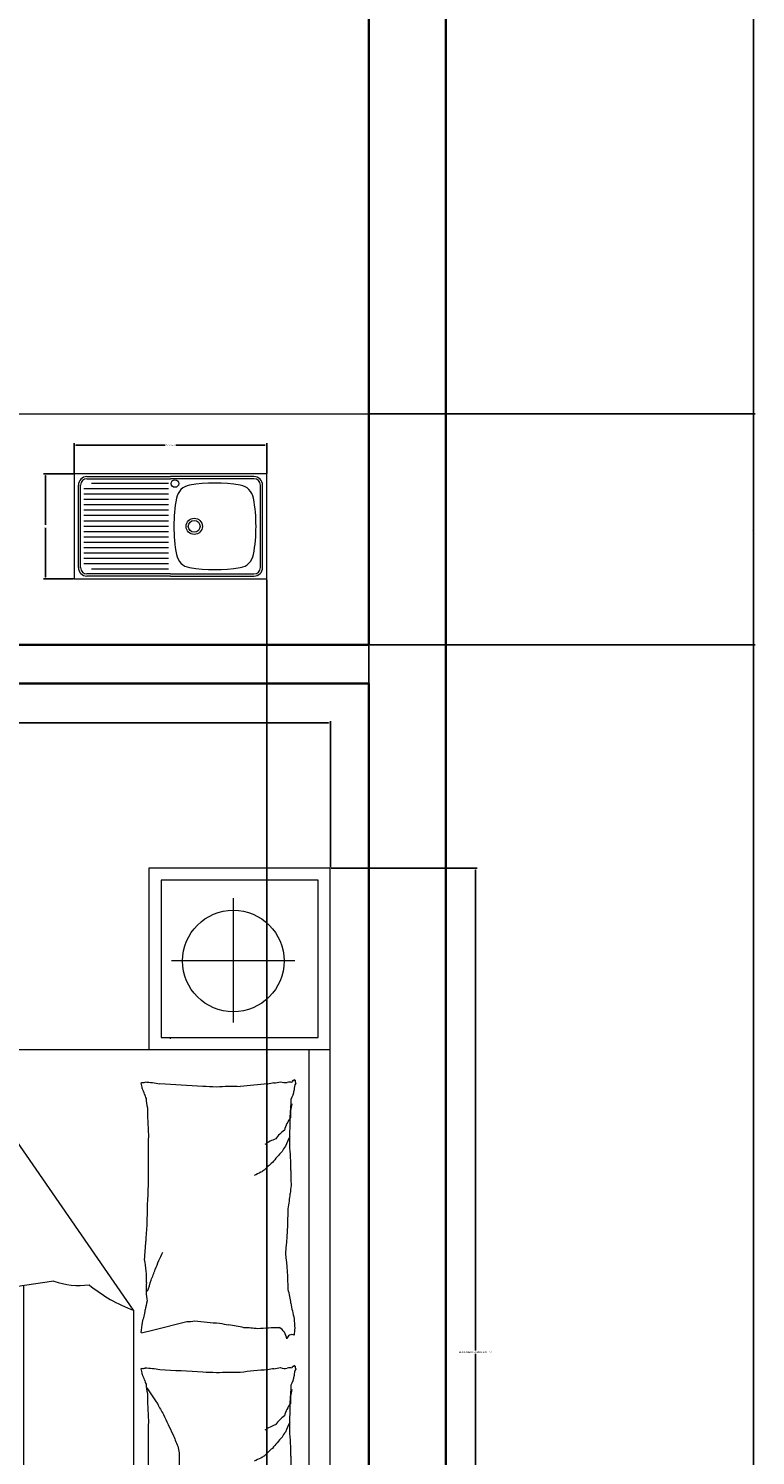
# Model space of a CAD drawing. Units: feet. Extents: x 1993 to 2298, y 2938 to 3641.
# Tile 7 of 11: x 2222 to 2298, y 3144 to 3293. Entities that reach past the tile are written whole.
import ezdxf

# ---------------------------------------------------------------- set-up
doc = ezdxf.new("R2010")
doc.units = ezdxf.units.FT
for name, color, linetype, lineweight in [('A-ANNO-DIMS', 2, 'Continuous', 18), ('A-FLOR-CASE', 8, 'Continuous', 18), ('A-FLOR-FIXT', 9, 'Continuous', 18), ('furniture', 8, 'Continuous', 18), ('WAL', 7, 'Continuous', 35)]:
    doc.layers.add(name, color=color, linetype=linetype, lineweight=lineweight)
doc.styles.add('DIM_FONT', font='SIMPLEX.shx', dxfattribs={"width": 0.8})
doc.styles.get("Standard").update_dxf_attribs({"font": 'arial.ttf'})
doc.dimstyles.get("Standard").update_dxf_attribs({"dimtxt": 0.18, "dimasz": 0.18, "dimexe": 0.18, "dimexo": 0.0625, "dimgap": 0.09, "dimtad": 0, "dimtih": 1, "dimtoh": 1, "dimdec": 4, "dimzin": 0, "dimdsep": 46, "dimtxsty": 'Standard', "dimcen": 0.09, "dimadec": 0, "dimazin": 0, "dimtfac": 1, "dimtdec": 4, "dimtofl": 0, "dimtmove": 0, "dimatfit": 3, "dimfxl": 1, "dimtolj": 1, "dimtzin": 0, "dimarcsym": 0})

# ---------------------------------------------------------------- blocks, each defined once
blk = doc.blocks.new('A$C79766A75')
for p, q in [((0.45, 1.9999), (0, 1.9999)), ((0, 1.9999), (0, 1.5499)), ((0.45, 1.5499), (0.45, 1.9999)), ((1.9506, 2), (0.4506, 2)), ((0.4506, 2), (0.4506, 0)), ((1.9506, 0), (1.9506, 2)), ((2.402, 1.9999), (1.952, 1.9999)), ((1.952, 1.9999), (1.952, 1.5499)), ((2.402, 1.5499), (2.402, 1.9999)), ((0.42, 1.9699), (0.03, 1.9699)), ((0.03, 1.9699), (0.03, 1.5799)), ((0.42, 1.5799), (0.42, 1.9699)), ((2.372, 1.9699), (1.982, 1.9699)), ((1.982, 1.9699), (1.982, 1.5799)), ((2.372, 1.5799), (2.372, 1.9699)), ((0.2304, 1.9125), (0.2304, 1.6061)), ((1.9506, 1.9476), (0.4506, 1.9476)), ((2.1824, 1.9125), (2.1824, 1.6061)), ((0.0743, 1.7595), (0.3834, 1.7595)), ((2.0263, 1.7595), (2.3354, 1.7595)), ((1.1461, 1.5617), (1.1254, 1.6443)), ((1.8553, 1.5617), (1.8346, 1.6443)), ((0.4234, 1.6034), (0.4228, 1.6034)), ((0.03, 1.5799), (0.42, 1.5799)), ((1.1536, 1.5317), (1.1461, 1.5617)), ((1.8628, 1.5317), (1.8553, 1.5617)), ((1.982, 1.5799), (2.372, 1.5799)), ((0, 1.5499), (0.45, 1.5499)), ((1.952, 1.5499), (2.402, 1.5499)), ((1.0972, 1.5115), (0.4791, 1.0841)), ((1.0972, 1.5115), (1.9048, 1.5115)), ((1.9248, 1.4915), (1.9248, 0.0322)), ((1.0383, 1.2184), (1.0246, 1.3138)), ((1.9048, 1.2389), (1.0354, 1.2389)), ((1.0365, 1.0883), (1.0383, 1.2184)), ((0.4791, 0.0622), (0.4791, 1.0841)), ((1.1731, 0.6316), (1.2523, 0.5276)), ((1.5696, 0.6317), (1.5559, 0.5286)), ((1.2523, 0.5276), (1.3274, 0.3973)), ((1.4223, 0.4407), (1.442, 0.5296)), ((1.5559, 0.5286), (1.5817, 0.4065)), ((1.6952, 0.4478), (1.7898, 0.4856)), ((1.7898, 0.4856), (1.8139, 0.4822)), ((1.4025, 0.3834), (1.4223, 0.4407)), ((1.6264, 0.355), (1.6952, 0.4478)), ((1.3274, 0.3973), (1.3452, 0.342)), ((1.5817, 0.4065), (1.6264, 0.355)), ((1.1139, 0.3597), (1.0779, 0.3397)), ((1.2167, 0.3736), (1.1139, 0.3597)), ((1.3452, 0.342), (1.2167, 0.3736)), ((1.3452, 0.342), (1.4025, 0.3834)), ((1.4034, 0.3558), (1.3803, 0.2995)), ((1.6264, 0.355), (1.4406, 0.3361)), ((1.5954, 0.2725), (1.6264, 0.355)), ((1.6264, 0.355), (1.6935, 0.3825)), ((1.6935, 0.3825), (1.7623, 0.379)), ((1.7623, 0.379), (1.8603, 0.3619)), ((1.8603, 0.3619), (1.8636, 0.3554)), ((1.2957, 0.2787), (1.3452, 0.342)), ((1.3452, 0.342), (1.3569, 0.2478)), ((1.4406, 0.3361), (1.3907, 0.3)), ((1.3803, 0.2995), (1.3626, 0.256)), ((1.3907, 0.3), (1.3787, 0.2914)), ((1.2305, 0.2313), (1.2957, 0.2787)), ((1.6161, 0.19), (1.5954, 0.2725)), ((1.1376, 0.2313), (1.2305, 0.2313)), ((1.3588, 0.2331), (1.3706, 0.1385)), ((1.6697, 0.1274), (1.6161, 0.19)), ((1.9048, 0.0122), (0.5291, 0.0122)), ((0.4506, 0), (1.9506, 0))]:
    blk.add_line(p, q)
for centre in [(0.2304, 1.7595), (2.1824, 1.7595)]:
    blk.add_circle(centre, 0.126)
for centre, radius, start, end in [((0.5232, 1.9139), 0.00342, 291.7883, 340.436), ((0.5246, 1.9378), 0.0251, 274.3025, 291.7883), ((0.5486, 1.9393), 0.0289, 239.3487, 274.3025), ((1.1179, 2.0719), 0.1611, 270, 278.4372), ((1.1592, 2.0011), 0.0904, 258.7276, 270), ((1.2325, 1.9139), 0.00342, 291.7883, 340.436), ((1.2338, 1.9378), 0.0251, 274.3025, 291.7883), ((1.2578, 1.9393), 0.0289, 239.3487, 274.3025), ((1.8271, 2.0719), 0.1611, 270, 278.4372), ((1.8684, 2.0011), 0.0904, 258.7276, 270), ((0.525, 1.9085), 0.00232, 340.436, 101.8931), ((0.5311, 1.9093), 0.00428, 201.9904, 281.8931), ((0.4996, 1.8889), 0.0328, 338.579, 8.1335), ((0.2896, 1.8253), 0.246, 8.1335, 12.1095), ((0.5465, 1.8994), 0.0156, 158.579, 201.9904), ((0.5458, 1.8568), 0.0539, 59.3487, 84.7408), ((0.546, 1.0829), 0.8208, 84.7408, 88.0921), ((0.6118, 2.0005), 0.0992, 254.0648, 274.2159), ((0.6775, 1.9817), 0.0992, 233.9136, 254.0648), ((0.6362, 0.406), 1.4943, 88.0921, 90.5757), ((0.7304, 1.9449), 0.0992, 216.1766, 233.9136), ((0.7737, 2.1075), 0.234, 242.7604, 249.1397), ((0.7591, 1.0293), 0.8732, 90.5757, 94.8018), ((0.738, 1.949), 0.0768, 231.6114, 242.7604), ((0.974, 2.1633), 0.3916, 226.1885, 231.6114), ((0.7631, 2.1919), 0.2897, 267.4614, 274.8018), ((0.8143, 2.0532), 0.1524, 259.8101, 267.4614), ((0.7515, 1.3747), 0.5293, 79.8101, 83.9133), ((0.8451, 0.8466), 1.049, 83.9133, 90), ((1.046, 1.2129), 0.6827, 90, 97.5469), ((1.1117, 1.6625), 0.2422, 97.5469, 105.744), ((1.0352, 2.2041), 0.3048, 278.4372, 285.744), ((1.171, 1.8579), 0.0342, 94.4002, 153.4195), ((1.1709, 1.9049), 0.0131, 153.4195, 258.7276), ((1.2342, 1.9085), 0.00232, 340.436, 101.8931), ((1.2404, 1.9093), 0.00428, 201.9904, 281.8931), ((1.2088, 1.8889), 0.0328, 338.579, 8.1335), ((0.9988, 1.8253), 0.246, 8.1335, 12.1095), ((1.2558, 1.8994), 0.0156, 158.579, 201.9904), ((1.2551, 1.8568), 0.0539, 59.3487, 84.7408), ((1.2552, 1.0829), 0.8208, 84.7408, 88.0921), ((1.3211, 2.0005), 0.0992, 254.0648, 274.2159), ((1.3868, 1.9817), 0.0992, 233.9136, 254.0648), ((1.3455, 0.406), 1.4943, 88.0921, 90.5757), ((1.4396, 1.9449), 0.0992, 216.1766, 233.9136), ((1.4829, 2.1075), 0.234, 242.7604, 249.1397), ((1.4683, 1.0293), 0.8732, 90.5757, 94.8018), ((1.4473, 1.949), 0.0768, 231.6114, 242.7604), ((1.6833, 2.1633), 0.3916, 226.1885, 231.6114), ((1.4724, 2.1919), 0.2897, 267.4614, 274.8018), ((1.5236, 2.0532), 0.1524, 259.8101, 267.4614), ((1.4607, 1.3747), 0.5293, 79.8101, 83.9133), ((1.5543, 0.8466), 1.049, 83.9133, 90), ((1.7552, 1.2129), 0.6827, 90, 97.5469), ((1.821, 1.6625), 0.2422, 97.5469, 105.744), ((1.7444, 2.2041), 0.3048, 278.4372, 285.744), ((1.8802, 1.8579), 0.0342, 94.4002, 153.4195), ((1.8802, 1.9049), 0.0131, 153.4195, 258.7276), ((0.7297, 1.8867), 0.1983, 187.6809, 192.1095), ((1.4472, 1.8987), 0.9131, 183.3687, 187.6809), ((0.7661, 1.8961), 0.0992, 198.4397, 216.1766), ((0.9057, 1.9982), 0.2252, 219.0349, 226.1885), ((1.6324, 1.8735), 0.4918, 180, 186.2324), ((1.4389, 1.8867), 0.1983, 187.6809, 192.1095), ((2.1565, 1.8987), 0.9131, 183.3687, 187.6809), ((1.4753, 1.8961), 0.0992, 198.4397, 216.1766), ((1.615, 1.9982), 0.2252, 219.0349, 226.1885), ((1.6908, 1.9123), 0.1399, 314.9024, 332.6012), ((1.7511, 1.9723), 0.1399, 297.2036, 314.9024), ((1.7896, 1.8667), 0.0526, 318.5571, 334.6449), ((1.784, 1.9167), 0.0899, 306.2641, 318.5571), ((2.3416, 1.8735), 0.4918, 180, 186.2324), ((0.7932, 1.8591), 0.0493, 208.3168, 219.0349), ((0.9392, 1.9062), 0.2002, 203.0028, 208.3168), ((1.3446, 1.7858), 0.204, 170.3156, 180), ((1.5025, 1.8591), 0.0493, 208.3168, 219.0349), ((1.6484, 1.9062), 0.2002, 203.0028, 208.3168), ((1.6554, 1.8529), 0.1399, 332.6012, 343.485), ((1.7653, 1.8132), 0.0562, 341.2201, 0), ((1.6307, 1.8895), 0.2056, 338.1851, 341.2201), ((1.6887, 1.8881), 0.1511, 334.6449, 338.1851), ((2.0538, 1.7858), 0.204, 170.3156, 180), ((1.2208, 1.7573), 0.6787, 178.3669, 183.3687), ((2.0027, 1.5994), 0.882, 167.8016, 170.3156), ((1.9301, 1.7573), 0.6787, 178.3669, 183.3687), ((1.6404, 1.8023), 0.1399, 343.485, 354.3689), ((1.73, 1.7719), 0.0915, 0, 14.6851), ((2.7119, 1.5994), 0.882, 167.8016, 170.3156), ((0.8192, 1.792), 0.3171, 347.8016, 351.9949), ((1.5284, 1.792), 0.3171, 347.8016, 351.9949), ((1.9066, 1.6447), 1.3652, 176.945, 178.3669), ((0.4711, 1.7556), 0.6588, 351.9949, 357.3351), ((2.6158, 1.6447), 1.3652, 176.945, 178.3669), ((1.1803, 1.7556), 0.6588, 351.9949, 357.3351), ((14.1519, 0.85), 13.6356, 176.49514, 176.94504), ((14.8612, 0.85), 13.6356, 176.49514, 176.94504), ((1.0578, 1.6474), 0.0677, 357.3351, 14.0452), ((1.767, 1.6474), 0.0677, 357.3351, 14.0452), ((0.7658, 2.8912), 1.4323, 294.3265, 296.4985), ((1.226, 2.0834), 0.5066, 290.6743, 294.3265), ((1.4305, 1.6796), 0.058, 274.0828, 290.6743), ((1.4679, 1.8969), 0.2721, 266.4448, 274.0828), ((0.8521, 1.5209), 0.3212, 170.0016, 176.4951), ((0.6583, 0.9067), 0.7387, 64.6889, 66.5156), ((0.7015, 0.888), 0.7387, 66.5156, 68.3423), ((0.7501, 0.8688), 0.7387, 68.3423, 70.572), ((1.5613, 1.5209), 0.3212, 170.0016, 176.4951), ((0.9025, 2.1618), 0.7286, 302.135, 305.8263), ((1.1895, 1.8508), 0.3126, 296.4985, 302.135), ((1.3675, 0.9067), 0.7387, 64.6889, 66.5156), ((1.4107, 0.888), 0.7387, 66.5156, 68.3423), ((1.4594, 0.8688), 0.7387, 68.3423, 70.572), ((0.513, 1.535), 0.0193, 350.0016, 16.6978), ((0.5322, 1.5304), 0.00132, 16.6978, 97.1204), ((0.5579, 1.4467), 0.0875, 97.1204, 106.2212), ((0.5822, 1.4654), 0.0767, 106.2212, 117.2841), ((0.5507, 1.5832), 0.0453, 282.869, 297.2841), ((0.5623, 1.6885), 0.1459, 273.574, 282.869), ((0.589, 2.7103), 1.164, 270.2865, 273.574), ((0.7584, 7.2662), 5.7185, 269.0296, 270.2865), ((0.9401, 4.9065), 3.3622, 267.3904, 269.0296), ((0.9811, 2.7573), 1.2165, 265.3824, 267.3904), ((0.8583, 0.139), 1.4048, 85.3824, 87.2509), ((1.0175, 1.3138), 0.2301, 87.2509, 101.5586), ((0.8043, 0.8497), 0.7387, 70.572, 72.8018), ((1.0449, 1.6886), 0.1459, 263.5659, 281.5586), ((1.1099, 1.6599), 0.1197, 252.6136, 263.5659), ((1.0587, 1.3144), 0.2297, 72.6136, 80.5159), ((1.108, 1.2635), 0.2708, 80.5159, 85.9171), ((1.1535, 1.5308), 0.000917, 85.9171, 194.0449), ((1.2222, 1.535), 0.0193, 350.0016, 16.6978), ((1.2414, 1.5304), 0.00132, 16.6978, 97.1204), ((1.2671, 1.4467), 0.0875, 97.1204, 106.2212), ((1.2914, 1.4654), 0.0767, 106.2212, 117.2841), ((1.2599, 1.5832), 0.0453, 282.869, 297.2841), ((1.2716, 1.6885), 0.1459, 273.574, 282.869), ((1.2982, 2.7103), 1.164, 270.2865, 273.574), ((1.4677, 7.2662), 5.7185, 269.0296, 270.2865), ((1.6493, 4.9065), 3.3622, 267.3904, 269.0296), ((1.6903, 2.7573), 1.2165, 265.3824, 267.3904), ((1.5676, 0.139), 1.4048, 85.3824, 87.2509), ((1.7268, 1.3138), 0.2301, 87.2509, 101.5586), ((1.5136, 0.8497), 0.7387, 70.572, 72.8018), ((1.7541, 1.6886), 0.1459, 263.5659, 281.5586), ((1.8192, 1.6599), 0.1197, 252.6136, 263.5659), ((1.7679, 1.3144), 0.2297, 72.6136, 80.5159), ((1.8172, 1.2635), 0.2708, 80.5159, 85.9171), ((1.8627, 1.5308), 0.000917, 85.9171, 194.0449), ((0.745, 1.6407), 0.3751, 320.3555, 339.8512), ((1.9048, 1.4915), 0.02, 0, 90), ((0.8556, 1.3759), 0.1801, 339.8512, 8.1356), ((1.9048, 1.2589), 0.02, 270, 0), ((-0.1888, 5.1029), 4.0646, 280.7276, 282.9255), ((0.7282, 1.1989), 0.0581, 262.2696, 280.7276), ((0.7833, 1.3309), 0.1942, 256.8096, 262.2696), ((0.2481, -1.3253), 2.5158, 76.8096, 78.3259), ((-0.0248, 2.8487), 1.8351, 285.9352, 287.7364), ((0.3872, 1.7415), 0.6574, 282.9255, 285.9352), ((0.3953, -1.4284), 2.588, 78.3259, 80.505), ((0.413, -2.64), 3.7801, 80.505, 82.308), ((1.1752, 0.6267), 0.0063, 166.7192, 233.4208), ((1.1734, 0.6272), 0.00443, 93.9484, 166.7192), ((1.163, 0.6103), 0.0142, 10.4074, 53.4208), ((1.1755, 0.5964), 0.0352, 69.6548, 93.9484), ((1.1011, 0.5989), 0.0771, 2.7286, 10.4074), ((1.1628, 0.6019), 0.0153, 345.4291, 2.7286), ((1.1669, 0.5731), 0.0601, 51.4146, 69.6548), ((1.2538, 0.682), 0.0792, 231.4146, 247.2931), ((1.5463, 1.3811), 0.8371, 247.2931, 249.8713), ((1.383, 0.7705), 0.2176, 307.2151, 313.5224), ((1.1426, 1.1456), 0.6605, 306.2163, 307.2151), ((1.7751, 0.3162), 0.3825, 126.2163, 127.5287), ((1.5806, 0.5924), 0.0452, 127.5287, 134.1274), ((1.5093, 0.6825), 0.0697, 308.8136, 314.1274), ((1.5706, 0.6318), 0.0127, 176.7545, 308.8136), ((1.5621, 0.59), 0.0359, 356.7545, 62.7098), ((0.9961, 0.6678), 0.194, 320.2995, 329.0944), ((0.8605, 0.749), 0.352, 329.0944, 333.1821), ((1.1396, 0.6079), 0.0393, 333.1821, 345.4291), ((3.0113, 5.3783), 5.0942, 249.8713, 250.9164), ((1.5435, 0.5526), 0.0458, 157.5838, 188.0492), ((1.4828, 0.5833), 0.0226, 324.1064, 8.0492), ((1.4519, 0.6426), 0.0774, 313.5224, 324.1064), ((0.2201, -2.1858), 3.0972, 62.7098, 63.5853), ((2.5711, 2.3551), 2.0162, 242.5001, 243.5853), ((1.2077, 0.4922), 0.081, 140.2995, 153.9265), ((2.374, 3.5362), 3.145, 250.9164, 253.3915), ((2.4089, 0.1204), 1.0054, 154.9471, 157.5838), ((4.5245, 5.9445), 6.1019, 242.15178, 242.50014), ((-0.9881, -4.647), 5.8383, 62.15178, 62.50792), ((3.0311, -0.112), 2.003, 162.1604, 164.7375), ((1.3115, 0.4414), 0.1965, 153.9265, 162.1604), ((2.9813, -0.2643), 1.6868, 152.9116, 154.9471), ((1.5084, 0.6341), 0.1166, 253.3915, 259.2634), ((1.5182, -0.068), 0.6236, 62.5079, 69.2514), ((1.7121, 0.0657), 0.43, 69.2514, 77.3748), ((1.8682, 0.4049), 0.063, 77.3748, 93.3881), ((1.8955, 0.5247), 0.0599, 256.9598, 273.3881), ((1.9257, 0.5082), 0.0509, 238.3083, 256.9598), ((2.8096, -0.3311), 1.5652, 150.064, 152.9116), ((1.8435, 0.4743), 0.0755, 310.5086, 333.6668), ((1.9279, 0.441), 0.0168, 130.5086, 180.9614), ((1.9201, 0.4587), 0.0058, 180.9614, 238.3083), ((2.6887, -0.0186), 1.6481, 164.7375, 166.159), ((-0.5166, 1.5491), 2.6619, 333.6668, 334.8268), ((0.5589, 0.5062), 0.5454, 343.6878, 346.159), ((1.2176, 0.4627), 0.2143, 330.064, 337.7645), ((1.3456, 0.5261), 0.5454, 339.2919, 341.7631), ((1.701, 0.4319), 0.1798, 334.8268, 339.2919), ((-1.4109, 1.284), 2.6619, 338.0627, 339.2227), ((0.9098, 0.4035), 0.1798, 339.2227, 343.6878), ((3.4079, -0.2212), 1.6481, 160.3416, 161.7631), ((0.9882, 0.3177), 0.0755, 314.9045, 338.0627), ((3.6966, -0.4634), 2.003, 157.7645, 160.3416), ((1.0533, 0.2524), 0.0168, 134.9045, 185.3572), ((1.0424, 0.2513), 0.0058, 185.3572, 242.7041), ((1.3694, 0.234), 0.0231, 107.1867, 157.7645), ((1.0631, 0.2914), 0.0509, 242.7041, 261.3557), ((1.0645, 0.3003), 0.0599, 261.3557, 277.784), ((1.0811, 0.1786), 0.063, 81.7707, 97.784), ((1.0286, -0.1846), 0.43, 73.6473, 81.7707), ((0.974, -0.3705), 0.6236, 66.9038, 73.6473), ((1.3465, 0.2383), 0.00467, 287.1867, 70.6201), ((1.3486, 0.2247), 0.0092, 70.6201, 94.2593), ((1.3563, 0.267), 0.034, 262.0178, 274.2593), ((1.4091, 0.4221), 0.1955, 255.1193, 262.0178), ((1.358, 0.0507), 0.1794, 75.1193, 82.3216), ((1.4096, 0.153), 0.0712, 82.3216, 94.5118), ((1.4285, 0.2893), 0.0663, 261.8784, 274.5118), ((1.4755, 0.332), 0.1166, 248.9957, 261.8784), ((2.7121, 3.1012), 3.145, 246.5205, 248.9957), ((2.4175, -0.1202), 1.0054, 160.6552, 161.9797), ((-1.0716, -5.1672), 5.8383, 66.54766, 66.9038), ((3.6805, 5.7866), 6.1019, 246.54766, 246.89602), ((1.505, 0.1766), 0.0458, 161.9797, 192.4451), ((1.856, 0.1288), 0.081, 135.9036, 149.5306), ((1.9797, 0.1108), 0.1965, 149.5306, 157.7645), ((2.0773, 2.0287), 2.0162, 246.896, 247.9812), ((0.1602, -2.7118), 3.0972, 67.1056, 67.9812), ((1.3914, 0.1905), 0.0774, 317.9183, 328.5023), ((1.4382, 0.1619), 0.0226, 328.5023, 12.4451), ((3.6993, 4.7998), 5.0942, 245.4754, 246.5205), ((1.4661, 0.3294), 0.352, 324.6985, 328.7862), ((1.6279, 0.2819), 0.194, 315.9036, 324.6985), ((1.3512, 0.1084), 0.0359, 1.1504, 67.1056), ((1.3997, 0.1094), 0.0127, 181.1504, 313.2095), ((1.4468, 0.0748), 0.0452, 131.9246, 138.5233), ((1.6722, -0.1762), 0.3825, 130.6122, 131.9246), ((0.9933, 0.6156), 0.6605, 310.6122, 311.611), ((1.2874, 0.2845), 0.2176, 311.611, 317.9183), ((2.051, 0.8725), 0.8371, 242.8972, 245.4754), ((1.7576, 0.1689), 0.0792, 227.0187, 242.8972), ((1.7345, 0.1188), 0.0153, 341.0332, 358.3327), ((1.6723, 0.1058), 0.0771, 358.3327, 6.0115), ((1.7162, 0.1388), 0.0393, 328.7862, 341.0332), ((1.3607, 0.1509), 0.0697, 313.2095, 318.5233), ((1.6963, 0.0438), 0.0601, 47.0187, 65.2589), ((1.737, 0.0526), 0.0352, 65.2589, 89.5525), ((1.7401, 0.0928), 0.0142, 6.0115, 49.0249), ((1.756, 0.0832), 0.00443, 89.5525, 162.3233), ((1.7602, 0.0924), 0.0063, 162.3233, 229.0249), ((0.5291, 0.0622), 0.05, 180, 270), ((1.9048, 0.0322), 0.02, 270, 0)]:
    blk.add_arc(centre, radius, start, end)
at = {"style": 'DIM_FONT', "text_generation_flag": 4, "width": 0.8, "flags": 9}
for tag in ['XSIZE', 'YSIZE']:
    blk.add_attdef(tag, (1.9506, 2), '', height=0.0005, rotation=180, dxfattribs=at)
blk = doc.blocks.new('A$C0C3933DC')
for p, q in [((0, 490), (0, 0)), ((900, 490), (0, 490)), ((59.5, 477.5), (450, 477.5)), ((59.5, 467.5), (450, 467.5)), ((840.5, 477.5), (450, 477.5)), ((840.5, 467.5), (450, 467.5)), ((900, 0), (900, 490)), ((19.5, 52.5), (19.5, 437.5)), ((29.5, 52.5), (29.5, 437.5)), ((441, 420), (45, 420)), ((441, 445), (80.7, 445)), ((870.5, 52.5), (870.5, 437.5)), ((880.5, 52.5), (880.5, 437.5)), ((441, 395), (45, 395)), ((441, 370), (45, 370)), ((441, 345), (45, 345)), ((441, 320), (45, 320)), ((441, 295), (45, 295)), ((441, 270), (45, 270)), ((441, 245), (45, 245)), ((441, 220), (45, 220)), ((441, 195), (45, 195)), ((441, 170), (45, 170)), ((441, 145), (45, 145)), ((441, 120), (45, 120)), ((441, 95), (45, 95)), ((441, 70), (45, 70)), ((0, 0), (900, 0)), ((450, 22.5), (59.5, 22.5)), ((450, 12.5), (59.5, 12.5)), ((441, 45), (80.7, 45)), ((450, 22.5), (840.5, 22.5)), ((450, 12.5), (840.5, 12.5))]:
    blk.add_line(p, q)
for centre, radius in [((471, 445), 17.5), ((561, 245), 38), ((561, 245), 27.5)]:
    blk.add_circle(centre, radius)
for centre, radius, start, end in [((59.5, 437.5), 40, 90, 180), ((59.5, 437.5), 30, 90, 180), ((840.5, 437.5), 40, 0, 90), ((840.5, 437.5), 30, 0, 90), ((551.5, 363.5), 75, 99.07872, 169.88522), ((658, -303), 750, 80.92128, 99.07872), ((764.5, 363.5), 75, 10.11478, 80.92128), ((1216, 245), 750, 169.88522, 190.11478), ((100, 245), 750, 349.88522, 10.11478), ((551.5, 126.5), 75, 190.11478, 260.92128), ((764.5, 126.5), 75, 279.07872, 349.88522), ((59.5, 52.5), 40, 180, 270), ((59.5, 52.5), 30, 180, 270), ((658, 793), 750, 260.92128, 279.07872), ((840.5, 52.5), 30, 270, 0), ((840.5, 52.5), 40, 270, 0)]:
    blk.add_arc(centre, radius, start, end)
blk = doc.blocks.new('*D30')
at = {"layer": 'A-ANNO-DIMS', "color": 0, "lineweight": -2, "transparency": 16777216}
for p, q in [((2253.83, 3205.36), (2269.02, 3205.36)), ((2268.84, 3205.18), (2268.84, 3155.29)), ((2268.84, 3105.04), (2268.84, 3154.93)), ((2253.83, 3104.86), (2269.02, 3104.86))]:
    blk.add_line(p, q, dxfattribs=at)
at = {"layer": 'A-ANNO-DIMS', "color": 0, "transparency": 16777216}
for points in [[(2268.81, 3205.18), (2268.87, 3205.18), (2268.84, 3205.36)], [(2268.81, 3105.04), (2268.87, 3105.04), (2268.84, 3104.86)]]:
    blk.add_solid(points, dxfattribs=at)
at = {"layer": 'Defpoints', "color": 0, "transparency": 16777216}
for p in [(2253.76, 3205.36), (2253.76, 3104.86), (2268.84, 3104.86)]:
    blk.add_point(p, dxfattribs=at)
at = {"layer": 'A-ANNO-DIMS', "color": 0, "transparency": 16777216, "insert": (2268.84, 3155.11), "char_height": 0.18, "attachment_point": 5}
blk.add_mtext('\\A1;BED & NIGHTSTANDS 100 TYP.', dxfattribs=at)
blk = doc.blocks.new('*D31')
at = {"layer": 'A-ANNO-DIMS', "color": 0, "lineweight": -2, "transparency": 16777216}
for p, q in [((2170.07, 3205.42), (2170.07, 3220.61)), ((2170.25, 3220.43), (2211.39, 3220.43)), ((2253.58, 3220.43), (2212.44, 3220.43)), ((2253.76, 3205.42), (2253.76, 3220.61))]:
    blk.add_line(p, q, dxfattribs=at)
at = {"layer": 'A-ANNO-DIMS', "color": 0, "transparency": 16777216}
for points in [[(2170.25, 3220.46), (2170.25, 3220.4), (2170.07, 3220.43)], [(2253.58, 3220.46), (2253.58, 3220.4), (2253.76, 3220.43)]]:
    blk.add_solid(points, dxfattribs=at)
at = {"layer": 'Defpoints', "color": 0, "transparency": 16777216}
for p in [(2253.76, 3220.43), (2170.07, 3205.36), (2253.76, 3205.36)]:
    blk.add_point(p, dxfattribs=at)
at = {"layer": 'A-ANNO-DIMS', "color": 0, "transparency": 16777216, "insert": (2211.92, 3220.43), "char_height": 0.18, "attachment_point": 5}
blk.add_mtext('\\A1;84 TYP.', dxfattribs=at)
blk = doc.blocks.new('*D52')
at = {"layer": 'A-ANNO-DIMS', "color": 0, "lineweight": -2, "transparency": 16777216}
for p, q in [((2227.15, 3246.35), (2227.15, 3249.47)), ((2227.33, 3249.29), (2236.6, 3249.29)), ((2246.97, 3249.29), (2237.7, 3249.29)), ((2247.15, 3246.35), (2247.15, 3249.47))]:
    blk.add_line(p, q, dxfattribs=at)
at = {"layer": 'A-ANNO-DIMS', "color": 0, "transparency": 16777216}
for points in [[(2227.33, 3249.32), (2227.33, 3249.26), (2227.15, 3249.29)], [(2246.97, 3249.32), (2246.97, 3249.26), (2247.15, 3249.29)]]:
    blk.add_solid(points, dxfattribs=at)
at = {"layer": 'Defpoints', "color": 0, "transparency": 16777216}
for p in [(2247.15, 3249.29), (2227.15, 3246.29), (2247.15, 3246.29)]:
    blk.add_point(p, dxfattribs=at)
at = {"layer": 'A-ANNO-DIMS', "color": 0, "transparency": 16777216, "insert": (2237.15, 3249.29), "char_height": 0.18, "attachment_point": 5}
blk.add_mtext('\\A1;SINK 20', dxfattribs=at)
blk = doc.blocks.new('*D53')
at = {"layer": 'A-ANNO-DIMS', "color": 0, "lineweight": -2, "transparency": 16777216}
for p, q in [((2227.09, 3246.29), (2223.97, 3246.29)), ((2224.15, 3246.11), (2224.15, 3241.02)), ((2224.15, 3235.58), (2224.15, 3240.66)), ((2227.09, 3235.4), (2223.97, 3235.4))]:
    blk.add_line(p, q, dxfattribs=at)
at = {"layer": 'A-ANNO-DIMS', "color": 0, "transparency": 16777216}
for points in [[(2224.12, 3246.11), (2224.18, 3246.11), (2224.15, 3246.29)], [(2224.12, 3235.58), (2224.18, 3235.58), (2224.15, 3235.4)]]:
    blk.add_solid(points, dxfattribs=at)
at = {"layer": 'Defpoints', "color": 0, "transparency": 16777216}
for p in [(2224.15, 3246.29), (2227.15, 3246.29), (2227.15, 3235.4)]:
    blk.add_point(p, dxfattribs=at)
at = {"layer": 'A-ANNO-DIMS', "color": 0, "transparency": 16777216, "insert": (2224.15, 3240.84), "char_height": 0.18, "attachment_point": 5}
blk.add_mtext('\\A1;11', dxfattribs=at)
blk = doc.blocks.new('*D55')
at = {"layer": 'A-ANNO-DIMS', "color": 0, "lineweight": -2, "transparency": 16777216}
for p, q in [((2265.82, 3608.53), (2297.9, 3608.53)), ((2297.72, 3608.35), (2297.72, 3308.72)), ((2297.72, 3008.71), (2297.72, 3308.35)), ((2265.82, 3008.53), (2297.9, 3008.53))]:
    blk.add_line(p, q, dxfattribs=at)
at = {"layer": 'A-ANNO-DIMS', "color": 0, "transparency": 16777216}
for points in [[(2297.69, 3608.35), (2297.75, 3608.35), (2297.72, 3608.53)], [(2297.69, 3008.71), (2297.75, 3008.71), (2297.72, 3008.53)]]:
    blk.add_solid(points, dxfattribs=at)
at = {"layer": 'Defpoints', "color": 0, "transparency": 16777216}
for p in [(2265.76, 3608.53), (2297.72, 3608.53), (2265.76, 3008.53)]:
    blk.add_point(p, dxfattribs=at)
at = {"layer": 'A-ANNO-DIMS', "color": 0, "transparency": 16777216, "insert": (2297.72, 3308.53), "char_height": 0.18, "attachment_point": 5}
blk.add_mtext('\\A1;600', dxfattribs=at)
blk = doc.blocks.new('*D61')
at = {"layer": 'A-ANNO-DIMS', "color": 0, "lineweight": -2, "transparency": 16777216}
for p, q in [((2257.82, 3252.53), (2297.9, 3252.53)), ((2297.72, 3252.35), (2297.72, 3240.71)), ((2297.72, 3228.71), (2297.72, 3240.35)), ((2257.82, 3228.53), (2297.9, 3228.53))]:
    blk.add_line(p, q, dxfattribs=at)
at = {"layer": 'A-ANNO-DIMS', "color": 0, "transparency": 16777216}
for points in [[(2297.69, 3252.35), (2297.75, 3252.35), (2297.72, 3252.53)], [(2297.69, 3228.71), (2297.75, 3228.71), (2297.72, 3228.53)]]:
    blk.add_solid(points, dxfattribs=at)
at = {"layer": 'Defpoints', "color": 0, "transparency": 16777216}
for p in [(2257.76, 3252.53), (2297.72, 3252.53), (2257.76, 3228.53)]:
    blk.add_point(p, dxfattribs=at)
at = {"layer": 'A-ANNO-DIMS', "color": 0, "transparency": 16777216, "insert": (2297.72, 3240.53), "char_height": 0.18, "attachment_point": 5}
blk.add_mtext('\\A1;24', dxfattribs=at)
blk = doc.blocks.new('*D66')
at = {"layer": 'A-ANNO-DIMS', "color": 0, "lineweight": -2, "transparency": 16777216}
for p, q in [((2247.15, 3235.34), (2247.15, 2937.86)), ((2257.76, 3228.47), (2257.76, 2937.86)), ((2247.33, 2938.03), (2252, 2938.03)), ((2257.58, 2938.03), (2252.91, 2938.03))]:
    blk.add_line(p, q, dxfattribs=at)
at = {"layer": 'A-ANNO-DIMS', "color": 0, "transparency": 16777216}
for points in [[(2247.33, 2938.07), (2247.33, 2938.01), (2247.15, 2938.03)], [(2257.58, 2938.07), (2257.58, 2938.01), (2257.76, 2938.03)]]:
    blk.add_solid(points, dxfattribs=at)
at = {"layer": 'Defpoints', "color": 0, "transparency": 16777216}
for p in [(2247.15, 3235.4), (2257.76, 3228.53), (2257.76, 2938.03)]:
    blk.add_point(p, dxfattribs=at)
at = {"layer": 'A-ANNO-DIMS', "color": 0, "transparency": 16777216, "insert": (2252.45, 2938.03), "char_height": 0.18, "attachment_point": 5}
blk.add_mtext('\\A1;10.608', dxfattribs=at)

msp = doc.modelspace()

# ---------------------------------------------------------------- linework, layer by layer
at = {"layer": 'A-FLOR-CASE'}
msp.add_line((2149.7583, 3252.5338), (2257.7583, 3252.5338), dxfattribs=at)
at = {"layer": 'WAL'}
for p, q in [((2265.7583, 3608.5338), (2265.7583, 3008.5338)), ((2257.7583, 3340.5338), (2257.7583, 3228.5338)), ((2145.7583, 3228.5338), (2257.7583, 3228.5338)), ((2149.7583, 3224.5338), (2257.7583, 3224.5338)), ((2257.7583, 3224.5338), (2257.7583, 3088.5338))]:
    msp.add_line(p, q, dxfattribs=at)

# ---------------------------------------------------------------- block references
at = {"layer": 'A-FLOR-FIXT', "xscale": 0.0222222222222278, "yscale": 0.0222222222222278, "zscale": 0.0222222222222278}
msp.add_blockref('A$C0C3933DC', (2227.1506, 3235.4), dxfattribs=at)
at = {"layer": 'furniture', "xscale": 41.83725109546206, "yscale": 41.83725109546206, "zscale": 41.83725109546206, "rotation": 270}
msp.add_blockref('A$C79766A75', (2170.0686, 3205.3572), dxfattribs=at)

# ---------------------------------------------------------------- dimensions: what is measured, and where the dimension line sits
at = {"layer": 'A-ANNO-DIMS'}
for base, p1, p2, picture, middle in [((2297.7233, 3608.5338), (2265.7583, 3008.5338), (2265.7583, 3608.5338), '*D55', (2297.7233, 3308.5338)), ((2297.7233, 3252.5338), (2257.7583, 3228.5338), (2257.7583, 3252.5338), '*D61', (2297.7233, 3240.5338)), ((2224.1506, 3246.2889), (2227.1506, 3235.4), (2227.1506, 3246.2889), '*D53', (2224.1506, 3240.8444))]:
    dim = msp.add_linear_dim(base=base, p1=p1, p2=p2, angle=90, dimstyle='Standard', override={"dimdec": 0, "dimlfac": 1, "dimrnd": 0, "dimzin": 0, "dimdsep": 46, "dimlunit": 2}, dxfattribs=at)
    dim.commit()
    dim.dimension.update_dxf_attribs({"geometry": picture, "text_midpoint": middle})
for base, p1, p2, text, picture, middle in [((2247.1506, 3249.2889), (2227.1506, 3246.2889), (2247.1506, 3246.2889), 'SINK <>', '*D52', (2237.1506, 3249.2889)), ((2253.764, 3220.431), (2170.0686, 3205.3572), (2253.764, 3205.3572), '<> TYP.', '*D31', (2211.9163, 3220.431))]:
    dim = msp.add_linear_dim(base=base, p1=p1, p2=p2, text=text, dimstyle='Standard', override={"dimdec": 0, "dimlfac": 1, "dimrnd": 0, "dimzin": 0, "dimdsep": 46, "dimlunit": 2}, dxfattribs=at)
    dim.commit()
    dim.dimension.update_dxf_attribs({"geometry": picture, "text_midpoint": middle})
dim = msp.add_linear_dim(base=(2257.7583, 2938.035), p1=(2247.1506, 3235.4), p2=(2257.7583, 3228.5338), dimstyle='Standard', override={"dimdec": 3, "dimlfac": 1, "dimrnd": 0, "dimzin": 0, "dimdsep": 46, "dimlunit": 2}, dxfattribs=at)
dim.commit()
dim.dimension.update_dxf_attribs({"geometry": '*D66', "text_midpoint": (2252.4545, 2938.035)})
dim = msp.add_linear_dim(base=(2268.8379, 3104.8648), p1=(2253.764, 3205.3572), p2=(2253.764, 3104.8648), angle=270, text='BED & NIGHTSTANDS <> TYP.', dimstyle='Standard', override={"dimdec": 0, "dimlfac": 1, "dimrnd": 0, "dimzin": 0, "dimdsep": 46, "dimlunit": 2}, dxfattribs=at)
dim.commit()
dim.dimension.update_dxf_attribs({"geometry": '*D30', "text_midpoint": (2268.8379, 3155.111)})

doc.saveas('drawing.dxf')
